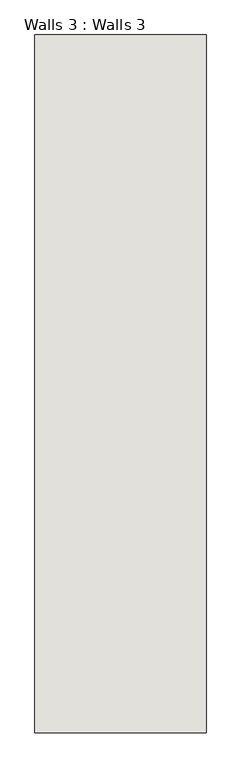
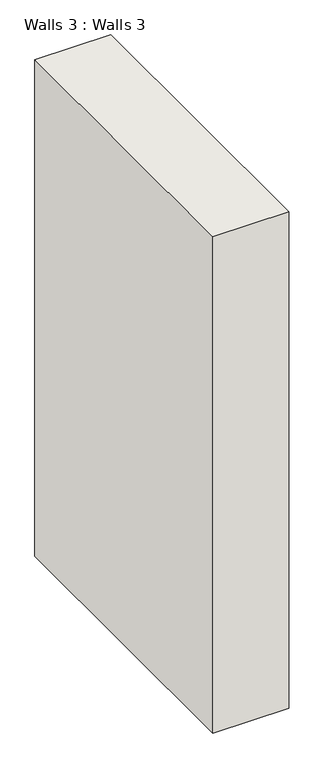
"""IFC4 building model written with IfcOpenShell, lengths in millimetres: wall geometry, Walls 3 : Walls 3."""

from ifc_helpers import new_model, si_unit, origin, origin_with_axes, place, context, project, spatial, polyline, outline, extrude, source, transform, mapped, element, save


def walls_3_walls_3_21c244ff(model_context):
    return source(origin(), model_context, "Body", "SweptSolid", [
        extrude(outline(polyline([(-5918.1391669, -5553.0913939), (-5918.1391669, -7911.1684063), (-6496.1866069, -7911.1684063), (-6496.1866069, -5553.0913939), (-5918.1391669, -5553.0913939)])), origin_with_axes(), (0.0, 0.0, 1.0), 4010.5440732),
    ])


if __name__ == "__main__":
    model = new_model("IFC4")
    model_context = context("Model", 3, world=origin())
    ifc_project = project(units=[si_unit("LENGTHUNIT", "METRE", prefix="MILLI")], contexts=[model_context])
    site = spatial("IfcSite", under=ifc_project)
    building = spatial("IfcBuilding", under=site)
    placement = place(None, origin())
    walls_3_walls_3_shape = walls_3_walls_3_21c244ff(model_context)
    element("IfcWall", 1, ObjectType="Walls 3 : Walls 3", at=placement, inside=building, context=model_context, shape_type="MappedRepresentation", body=[
        mapped(walls_3_walls_3_shape, transform((0.0, 0.0, 0.0), x_axis=(1.0, 0.0, 0.0), y_axis=(0.0, 1.0, 0.0), z_axis=(0.0, 0.0, 1.0))),
    ])
    save(model, "model.ifc")

# Revit data of these elements
# Element 1 (IfcWall, "Walls 3 : Walls 3")
#   Materials on its faces: "Default Wall"
# Materials
#   "Default Wall": colour RGB 80 80 80, transparency 0
